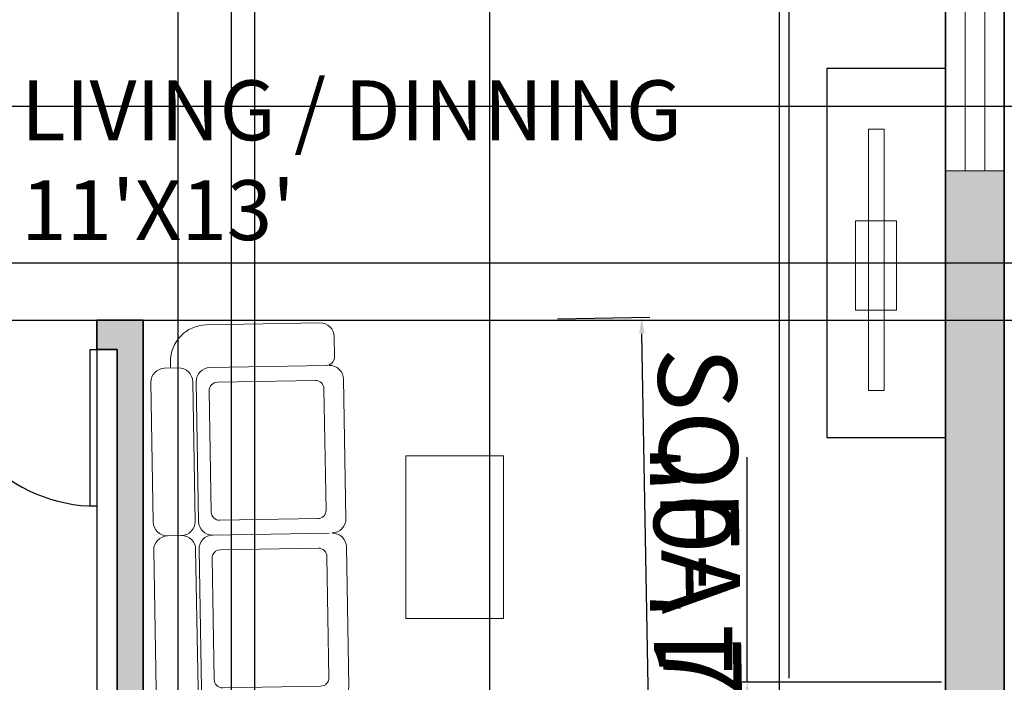
# Model space of a CAD drawing. Units: inches. Extents: x 1810 to 2254, y 313 to 1026.
# Tile 4 of 7: x 1988 to 2139, y 559 to 661. Entities that reach past the tile are written whole.
import ezdxf

# ---------------------------------------------------------------- set-up
doc = ezdxf.new("R2010")
doc.units = ezdxf.units.IN
for name, color, linetype, lineweight in [('A-ANNO-DIMS', 2, 'Continuous', 18), ('A-AREA-IDEN', 7, 'Continuous', 25), ('A-DOOR', 4, 'Continuous', 25), ('A-EQPM', 9, 'Continuous', 18), ('A-FLOR-CASE', 8, 'Continuous', 25), ('A-FURN', 8, 'Continuous', 18), ('A-GLAZ', 4, 'Continuous', 18), ('A-WALL', 7, 'Continuous', 35)]:
    doc.layers.add(name, color=color, linetype=linetype, lineweight=lineweight)
doc.layers.add('A-WALL-PATT', color=252, linetype='Continuous', lineweight=13, true_color=0x939598)
doc.styles.get("Standard").update_dxf_attribs({"font": 'arial.ttf'})
doc.dimstyles.new('ISO-25', dxfattribs={"dimtxt": 12, "dimasz": 2.5, "dimexe": 1.25, "dimexo": 0.625, "dimtad": 1, "dimdec": 1, "dimlunit": 4, "dimtxsty": 'Standard', "dimcen": 2.5, "dimadec": 0, "dimazin": 0, "dimtfac": 1, "dimtdec": 1, "dimtmove": 0, "dimatfit": 3, "dimfxl": 1, "dimarcsym": 0})

# ---------------------------------------------------------------- blocks, each defined once
blk = doc.blocks.new('A$C611E44E9')
for p, q in [((0.6611, 1.4447), (0.2101, 1.4447)), ((0.7111, 1.3223), (0.7111, 1.3947)), ((0.1084, 1.2927), (0.0584, 1.2927)), ((0.0584, 1.2924), (0.1084, 1.2924)), ((0.6811, 1.2924), (0.2205, 1.2924)), ((0.6811, 1.2924), (0.2205, 1.2924)), ((0.6811, 1.2922), (0.2205, 1.2922)), ((0.0084, 1.2424), (0.0084, 0.7424)), ((0.1584, 1.2424), (0.1584, 0.7424)), ((0.1705, 1.2422), (0.1705, 0.7424)), ((0.2465, 1.2392), (0.6374, 1.2392)), ((0.7418, 0.7424), (0.7418, 1.2422)), ((0.2165, 0.7749), (0.2165, 1.2092)), ((0.6674, 1.2092), (0.6674, 0.7749)), ((0.6374, 0.7449), (0.2465, 0.7449)), ((0.1224, 0.6827), (0.05, 0.6827)), ((0.1084, 0.6927), (0.0584, 0.6927)), ((0.0584, 0.6924), (0.1084, 0.6924)), ((0.2024, 0.6896), (0.7021, 0.6896)), ((0.6373, 0.6924), (0.2205, 0.6924)), ((0.6373, 0.6924), (0.2205, 0.6924)), ((0.8021, 0.6896), (1.3018, 0.6896)), ((1.4021, 0.6896), (1.9018, 0.6896)), ((0.1524, 0.6527), (0.1524, 0.2121)), ((1.982, 0.6589), (2.0543, 0.6589)), ((0, 0.6327), (0, 0.2017)), ((0.6691, 0.6192), (0.2348, 0.6192)), ((0.7521, 0.6289), (0.7521, 0.2121)), ((0.7521, 0.6289), (0.7521, 0.2121)), ((1.2688, 0.6192), (0.8345, 0.6192)), ((1.3521, 0.6289), (1.3521, 0.2121)), ((1.3521, 0.6289), (1.3521, 0.2121)), ((1.8688, 0.6192), (1.4345, 0.6192)), ((1.9518, 0.6289), (1.9518, 0.2121)), ((1.952, 0.6289), (1.952, 0.2121)), ((2.1043, 0.6089), (2.1043, 0.2017)), ((0.2048, 0.5892), (0.2048, 0.2381)), ((0.6991, 0.2381), (0.6991, 0.5892)), ((0.8045, 0.5892), (0.8045, 0.2381)), ((1.2988, 0.2381), (1.2988, 0.5892)), ((1.4045, 0.5892), (1.4045, 0.2381)), ((1.8988, 0.2381), (1.8988, 0.5892)), ((0.2348, 0.2081), (0.6691, 0.2081)), ((0.8345, 0.2081), (1.2688, 0.2081)), ((1.4345, 0.2081), (1.8688, 0.2081)), ((0.7021, 0.1621), (0.2024, 0.1621)), ((0.7024, 0.15), (0.2024, 0.15)), ((1.3018, 0.1621), (0.8021, 0.1621)), ((1.3021, 0.15), (0.8021, 0.15)), ((1.9018, 0.1621), (1.4021, 0.1621)), ((1.9021, 0.15), (1.4021, 0.15)), ((0.13, 0.0717), (0.15, 0.0717)), ((0.1524, 0.05), (0.1524, 0.1)), ((0.7521, 0.05), (0.7521, 0.1)), ((0.7524, 0.1), (0.7524, 0.05)), ((1.3521, 0.05), (1.3521, 0.1)), ((1.3524, 0.1), (1.3524, 0.05)), ((1.952, 0.05), (1.952, 0.1)), ((1.9521, 0.1), (1.9521, 0.05)), ((1.9743, 0.0717), (1.9543, 0.0717)), ((0.7024, 0), (0.2024, 0)), ((1.3021, 0), (0.8021, 0)), ((1.9021, 0), (1.4021, 0))]:
    blk.add_line(p, q)
for centre, radius, start, end in [((0.2101, 1.3147), 0.13, 90, 189.8614), ((0.6611, 1.3947), 0.05, 0, 90), ((0.6811, 1.3223), 0.03, 270, 0), ((0.0584, 1.2424), 0.05, 90, 180), ((0.1084, 1.2424), 0.05, 0, 90), ((0.2205, 1.2422), 0.05, 90, 180), ((0.6918, 1.2422), 0.05, 0, 90), ((0.2465, 1.2092), 0.03, 90, 180), ((0.6374, 1.2092), 0.03, 0, 90), ((0.0584, 0.7424), 0.05, 180, 270), ((0.1084, 0.7424), 0.05, 270, 0), ((0.2205, 0.7424), 0.05, 180, 270), ((0.2465, 0.7749), 0.03, 180, 270), ((0.6374, 0.7749), 0.03, 270, 0), ((0.653, 0.796), 0.1037, 267.2489, 328.8794), ((0.05, 0.6327), 0.05, 90, 180), ((0.1224, 0.6527), 0.03, 0, 90), ((0.1981, 0.6441), 0.0458, 84.6649, 178.9903), ((0.7021, 0.6396), 0.05, 0, 90), ((0.8021, 0.6396), 0.05, 90, 180), ((1.3018, 0.6396), 0.05, 0, 90), ((1.4021, 0.6396), 0.05, 90, 180), ((1.9018, 0.6396), 0.05, 0, 90), ((1.982, 0.6289), 0.03, 90, 180), ((2.0543, 0.6089), 0.05, 0, 90), ((0.2348, 0.5892), 0.03, 90, 180), ((0.6691, 0.5892), 0.03, 0, 90), ((0.8345, 0.5892), 0.03, 90, 180), ((1.2688, 0.5892), 0.03, 0, 90), ((1.4345, 0.5892), 0.03, 90, 180), ((1.8688, 0.5892), 0.03, 0, 90), ((0.2024, 0.2121), 0.05, 180, 270), ((0.2348, 0.2381), 0.03, 180, 270), ((0.6691, 0.2381), 0.03, 270, 0), ((0.7021, 0.2121), 0.05, 270, 0), ((0.8021, 0.2121), 0.05, 180, 270), ((0.8345, 0.2381), 0.03, 180, 270), ((1.2688, 0.2381), 0.03, 270, 0), ((1.3018, 0.2121), 0.05, 270, 0), ((1.4021, 0.2121), 0.05, 180, 270), ((1.4345, 0.2381), 0.03, 180, 270), ((1.8688, 0.2381), 0.03, 270, 0), ((1.9018, 0.2121), 0.05, 270, 0), ((0.13, 0.2017), 0.13, 180, 270), ((1.9743, 0.2017), 0.13, 270, 0), ((0.2024, 0.1), 0.05, 90, 180), ((0.7024, 0.1), 0.05, 0, 90), ((0.8021, 0.1), 0.05, 90, 180), ((1.3021, 0.1), 0.05, 0, 90), ((1.4021, 0.1), 0.05, 90, 180), ((1.9021, 0.1), 0.05, 0, 90), ((0.2024, 0.05), 0.05, 180, 270), ((0.7024, 0.05), 0.05, 270, 0), ((0.8021, 0.05), 0.05, 180, 270), ((1.3021, 0.05), 0.05, 270, 0), ((1.4021, 0.05), 0.05, 180, 270), ((1.9021, 0.05), 0.05, 270, 0)]:
    blk.add_arc(centre, radius, start, end)
blk = doc.blocks.new('*U16')
for p, q in [((0, 0), (0, -6)), ((40, 0), (40, -6))]:
    blk.add_line(p, q)
blk.add_lwpolyline([(0, 0), (0, 40), (1.75, 40), (1.75, 0)], close=True)
blk.add_arc((0, 0), 40, 0, 90)
blk = doc.blocks.new('*D23')
at = {"layer": 'A-ANNO-DIMS', "color": 0, "lineweight": -2, "transparency": 16777216}
for p, q in [((2130.99, 851.61), (2253.63, 851.61)), ((2252.38, 849.11), (2252.38, 437.11)), ((2130.99, 434.61), (2253.63, 434.61))]:
    blk.add_line(p, q, dxfattribs=at)
at = {"layer": 'A-ANNO-DIMS', "color": 0, "transparency": 16777216}
for points in [[(2251.96, 849.11), (2252.8, 849.11), (2252.38, 851.61)], [(2251.96, 437.11), (2252.8, 437.11), (2252.38, 434.61)]]:
    blk.add_solid(points, dxfattribs=at)
at = {"layer": 'Defpoints', "color": 0, "transparency": 16777216}
for p in [(2130.36, 851.61), (2130.36, 434.61), (2252.38, 434.61)]:
    blk.add_point(p, dxfattribs=at)
at = {"layer": 'A-ANNO-DIMS', "color": 0, "transparency": 16777216, "insert": (2245.62, 643.11), "char_height": 12, "attachment_point": 5, "rotation": 90}
blk.add_mtext('34\'-9"', dxfattribs=at)
blk = doc.blocks.new('WIN-36IN-WALL9')
for p, q in [((0, 9), (0, 0)), ((36, 9), (36, 0)), ((0, 6), (36, 6)), ((0, 3), (36, 3))]:
    blk.add_line(p, q)
blk = doc.blocks.new('*D44')
at = {"layer": 'A-ANNO-DIMS', "color": 0, "lineweight": -2, "transparency": 16777216}
for p, q in [((2070.88, 614.82), (2085.02, 615.06)), ((2085.29, 527.43), (2083.81, 612.54)), ((2072.44, 524.71), (2086.58, 524.96))]:
    blk.add_line(p, q, dxfattribs=at)
at = {"layer": 'A-ANNO-DIMS', "color": 0, "transparency": 16777216}
for points in [[(2084.23, 612.55), (2083.4, 612.54), (2083.77, 615.04)], [(2085.7, 527.44), (2084.87, 527.43), (2085.33, 524.93)]]:
    blk.add_solid(points, dxfattribs=at)
at = {"layer": 'Defpoints', "color": 0, "transparency": 16777216}
for p in [(2070.25, 614.81), (2083.77, 615.04), (2071.81, 524.7)]:
    blk.add_point(p, dxfattribs=at)
at = {"layer": 'A-ANNO-DIMS', "color": 0, "transparency": 16777216, "insert": (2091.38, 570.11), "char_height": 12, "attachment_point": 5, "rotation": 270.9916}
blk.add_mtext('SOFA 7\'-6"', dxfattribs=at)
blk = doc.blocks.new('*D54')
at = {"layer": 'A-ANNO-DIMS', "color": 0, "lineweight": -2, "transparency": 16777216}
for p, q in [((2130.99, 715.11), (2162.01, 715.11)), ((2160.76, 712.61), (2160.76, 676.02)), ((2130.99, 673.52), (2162.01, 673.52)), ((2160.76, 673.52), (2160.76, 609.92))]:
    blk.add_line(p, q, dxfattribs=at)
at = {"layer": 'A-ANNO-DIMS', "color": 0, "transparency": 16777216}
for points in [[(2160.35, 712.61), (2161.18, 712.61), (2160.76, 715.11)], [(2160.35, 676.02), (2161.18, 676.02), (2160.76, 673.52)]]:
    blk.add_solid(points, dxfattribs=at)
at = {"layer": 'Defpoints', "color": 0, "transparency": 16777216}
for p in [(2130.36, 715.11), (2130.36, 673.52), (2160.76, 673.52)]:
    blk.add_point(p, dxfattribs=at)
at = {"layer": 'A-ANNO-DIMS', "color": 0, "transparency": 16777216, "insert": (2153.93, 640.47), "char_height": 12, "attachment_point": 5, "rotation": 90}
blk.add_mtext('3\'-5 1/2"', dxfattribs=at)
blk = doc.blocks.new('*D57')
at = {"layer": 'A-ANNO-DIMS', "color": 0, "lineweight": -2, "transparency": 16777216}
for p, q in [((2104.86, 718.99), (2104.86, 323.71)), ((2130.36, 718.99), (2130.36, 323.71)), ((2107.36, 324.96), (2127.86, 324.96)), ((2130.36, 324.96), (2194.18, 324.96))]:
    blk.add_line(p, q, dxfattribs=at)
at = {"layer": 'A-ANNO-DIMS', "color": 0, "transparency": 16777216}
for points in [[(2107.36, 325.38), (2107.36, 324.55), (2104.86, 324.96)], [(2127.86, 325.38), (2127.86, 324.55), (2130.36, 324.96)]]:
    blk.add_solid(points, dxfattribs=at)
at = {"layer": 'Defpoints', "color": 0, "transparency": 16777216}
for p in [(2104.86, 719.61), (2130.36, 719.61), (2130.36, 324.96)]:
    blk.add_point(p, dxfattribs=at)
at = {"layer": 'A-ANNO-DIMS', "color": 0, "transparency": 16777216, "insert": (2163.52, 331.79), "char_height": 12, "attachment_point": 5}
blk.add_mtext('2\'-1 1/2"', dxfattribs=at)
blk = doc.blocks.new('*D59')
at = {"layer": 'A-ANNO-DIMS', "color": 0, "lineweight": -2, "transparency": 16777216}
for p, q in [((2024.44, 714.49), (2024.44, 323.71)), ((2060.44, 714.49), (2060.44, 323.71)), ((2026.94, 324.96), (2057.94, 324.96))]:
    blk.add_line(p, q, dxfattribs=at)
at = {"layer": 'A-ANNO-DIMS', "color": 0, "transparency": 16777216}
for points in [[(2026.94, 325.38), (2026.94, 324.55), (2024.44, 324.96)], [(2057.94, 325.38), (2057.94, 324.55), (2060.44, 324.96)]]:
    blk.add_solid(points, dxfattribs=at)
at = {"layer": 'Defpoints', "color": 0, "transparency": 16777216}
for p in [(2024.44, 715.11), (2060.44, 715.11), (2060.44, 324.96)]:
    blk.add_point(p, dxfattribs=at)
at = {"layer": 'A-ANNO-DIMS', "color": 0, "transparency": 16777216, "insert": (2042.44, 331.72), "char_height": 12, "attachment_point": 5}
blk.add_mtext('3\'-0"', dxfattribs=at)
blk = doc.blocks.new('*D61')
at = {"layer": 'A-ANNO-DIMS', "color": 0, "lineweight": -2, "transparency": 16777216}
for p, q in [((2106.36, 559.74), (2106.36, 892.26)), ((2130.36, 559.74), (2130.36, 892.26)), ((2108.86, 891.01), (2127.86, 891.01)), ((2130.36, 891.01), (2166.22, 891.01))]:
    blk.add_line(p, q, dxfattribs=at)
at = {"layer": 'A-ANNO-DIMS', "color": 0, "transparency": 16777216}
for points in [[(2108.86, 891.43), (2108.86, 890.6), (2106.36, 891.01)], [(2127.86, 891.43), (2127.86, 890.6), (2130.36, 891.01)]]:
    blk.add_solid(points, dxfattribs=at)
at = {"layer": 'Defpoints', "color": 0, "transparency": 16777216}
for p in [(2130.36, 891.01), (2106.36, 559.11), (2130.36, 559.11)]:
    blk.add_point(p, dxfattribs=at)
at = {"layer": 'A-ANNO-DIMS', "color": 0, "transparency": 16777216, "insert": (2149.54, 897.76), "char_height": 12, "attachment_point": 5}
blk.add_mtext('2\'-0"', dxfattribs=at)
blk = doc.blocks.new('*D63')
at = {"layer": 'A-ANNO-DIMS', "color": 0, "lineweight": -2, "transparency": 16777216}
for p, q in [((2169.76, 679.36), (2169.76, 715.21)), ((1973.49, 679.36), (2171.01, 679.36)), ((2169.76, 649.92), (2169.76, 676.86)), ((1973.49, 647.42), (2171.01, 647.42))]:
    blk.add_line(p, q, dxfattribs=at)
at = {"layer": 'A-ANNO-DIMS', "color": 0, "transparency": 16777216}
for points in [[(2169.35, 676.86), (2170.18, 676.86), (2169.76, 679.36)], [(2169.35, 649.92), (2170.18, 649.92), (2169.76, 647.42)]]:
    blk.add_solid(points, dxfattribs=at)
at = {"layer": 'Defpoints', "color": 0, "transparency": 16777216}
for p in [(1972.86, 679.36), (2169.76, 679.36), (1972.86, 647.42)]:
    blk.add_point(p, dxfattribs=at)
at = {"layer": 'A-ANNO-DIMS', "color": 0, "transparency": 16777216, "insert": (2163.01, 698.54), "char_height": 12, "attachment_point": 5, "rotation": 90}
blk.add_mtext('2\'-8"', dxfattribs=at)
blk = doc.blocks.new('*D64')
at = {"layer": 'A-ANNO-DIMS', "color": 0, "lineweight": -2, "transparency": 16777216}
for p, q in [((2169.76, 623.42), (2169.76, 659.07)), ((1973.49, 623.42), (2171.01, 623.42)), ((2169.76, 617.11), (2169.76, 620.92)), ((1973.49, 614.61), (2171.01, 614.61))]:
    blk.add_line(p, q, dxfattribs=at)
at = {"layer": 'A-ANNO-DIMS', "color": 0, "transparency": 16777216}
for points in [[(2169.35, 620.92), (2170.18, 620.92), (2169.76, 623.42)], [(2169.35, 617.11), (2170.18, 617.11), (2169.76, 614.61)]]:
    blk.add_solid(points, dxfattribs=at)
at = {"layer": 'Defpoints', "color": 0, "transparency": 16777216}
for p in [(1972.86, 623.42), (2169.76, 623.42), (1972.86, 614.61)]:
    blk.add_point(p, dxfattribs=at)
at = {"layer": 'A-ANNO-DIMS', "color": 0, "transparency": 16777216, "insert": (2163.01, 642.49), "char_height": 12, "attachment_point": 5, "rotation": 90}
blk.add_mtext('0\'-9"', dxfattribs=at)
blk = doc.blocks.new('*D66')
at = {"layer": 'A-ANNO-DIMS', "color": 0, "lineweight": -2, "transparency": 16777216}
for p, q in [((1976.27, 609.49), (1976.27, 323.71)), ((2000.27, 609.49), (2000.27, 323.71)), ((1978.77, 324.96), (1997.77, 324.96)), ((2000.27, 324.96), (2036.12, 324.96))]:
    blk.add_line(p, q, dxfattribs=at)
at = {"layer": 'A-ANNO-DIMS', "color": 0, "transparency": 16777216}
for points in [[(1978.77, 325.38), (1978.77, 324.55), (1976.27, 324.96)], [(1997.77, 325.38), (1997.77, 324.55), (2000.27, 324.96)]]:
    blk.add_solid(points, dxfattribs=at)
at = {"layer": 'Defpoints', "color": 0, "transparency": 16777216}
for p in [(1976.27, 610.11), (2000.27, 610.11), (2000.27, 324.96)]:
    blk.add_point(p, dxfattribs=at)
at = {"layer": 'A-ANNO-DIMS', "color": 0, "transparency": 16777216, "insert": (2019.45, 331.72), "char_height": 12, "attachment_point": 5}
blk.add_mtext('2\'-0"', dxfattribs=at)
blk = doc.blocks.new('*D67')
at = {"layer": 'A-ANNO-DIMS', "color": 0, "lineweight": -2, "transparency": 16777216}
for p, q in [((1976.68, 714.49), (1976.68, 323.71)), ((2012.68, 714.49), (2012.68, 323.71)), ((1979.18, 324.96), (2010.18, 324.96))]:
    blk.add_line(p, q, dxfattribs=at)
at = {"layer": 'A-ANNO-DIMS', "color": 0, "transparency": 16777216}
for points in [[(1979.18, 325.38), (1979.18, 324.55), (1976.68, 324.96)], [(2010.18, 325.38), (2010.18, 324.55), (2012.68, 324.96)]]:
    blk.add_solid(points, dxfattribs=at)
at = {"layer": 'Defpoints', "color": 0, "transparency": 16777216}
for p in [(1976.68, 715.11), (2012.68, 715.11), (2012.68, 324.96)]:
    blk.add_point(p, dxfattribs=at)
at = {"layer": 'A-ANNO-DIMS', "color": 0, "transparency": 16777216, "insert": (1994.68, 331.72), "char_height": 12, "attachment_point": 5}
blk.add_mtext('3\'-0"', dxfattribs=at)
blk = doc.blocks.new('*D68')
at = {"layer": 'A-ANNO-DIMS', "color": 0, "lineweight": -2, "transparency": 16777216}
for p, q in [((2020.86, 826.99), (2020.86, 323.71)), ((2104.86, 826.99), (2104.86, 323.71)), ((2023.36, 324.96), (2102.36, 324.96))]:
    blk.add_line(p, q, dxfattribs=at)
at = {"layer": 'A-ANNO-DIMS', "color": 0, "transparency": 16777216}
for points in [[(2023.36, 325.38), (2023.36, 324.55), (2020.86, 324.96)], [(2102.36, 325.38), (2102.36, 324.55), (2104.86, 324.96)]]:
    blk.add_solid(points, dxfattribs=at)
at = {"layer": 'Defpoints', "color": 0, "transparency": 16777216}
for p in [(2020.86, 827.61), (2104.86, 827.61), (2104.86, 324.96)]:
    blk.add_point(p, dxfattribs=at)
at = {"layer": 'A-ANNO-DIMS', "color": 0, "transparency": 16777216, "insert": (2062.86, 331.72), "char_height": 12, "attachment_point": 5}
blk.add_mtext('7\'-0"', dxfattribs=at)
blk = doc.blocks.new('*D75')
at = {"layer": 'A-ANNO-DIMS', "color": 0, "lineweight": -2, "transparency": 16777216}
for p, q in [((2099.96, 559.11), (2099.96, 593.63)), ((2129.74, 559.11), (2098.71, 559.11)), ((2099.96, 549.61), (2099.96, 556.61)), ((2129.74, 547.11), (2098.71, 547.11))]:
    blk.add_line(p, q, dxfattribs=at)
at = {"layer": 'A-ANNO-DIMS', "color": 0, "transparency": 16777216}
for points in [[(2099.55, 556.61), (2100.38, 556.61), (2099.96, 559.11)], [(2099.55, 549.61), (2100.38, 549.61), (2099.96, 547.11)]]:
    blk.add_solid(points, dxfattribs=at)
at = {"layer": 'Defpoints', "color": 0, "transparency": 16777216}
for p in [(2099.96, 559.11), (2130.36, 559.11), (2130.36, 547.11)]:
    blk.add_point(p, dxfattribs=at)
at = {"layer": 'A-ANNO-DIMS', "color": 0, "transparency": 16777216, "insert": (2093.21, 577.62), "char_height": 12, "attachment_point": 5, "rotation": 90}
blk.add_mtext('1\'-0"', dxfattribs=at)

msp = doc.modelspace()

# ---------------------------------------------------------------- hatches: boundary and pattern name
at = {"layer": 'A-WALL-PATT'}
h = msp.add_hatch(color=256, dxfattribs=at)
h.dxf.hatch_style = 1
h.paths.add_polyline_path([(1943.78, 860.61), (1875.36, 860.61), (1875.36, 706.11), (1884.36, 706.11), (1884.36, 715.11), (1968.36, 715.11), (1968.36, 703.36), (1971.96, 703.36), (1972.86, 703.36), (1972.86, 715.11), (1976.68, 715.11), (1976.68, 719.61), (1884.36, 719.61), (1884.36, 851.61), (1943.73, 851.61)])
h.paths.add_polyline_path([(2048.15, 860.61), (1979.78, 860.61), (1979.73, 851.61), (2016.36, 851.61), (2016.36, 719.61), (2012.68, 719.61), (2012.68, 716.01), (2012.68, 715.11), (2024.44, 715.11), (2024.44, 719.61), (2020.86, 719.61), (2020.86, 851.61), (2048.15, 851.61)])
h.paths.add_polyline_path([(2139.36, 860.61), (2084.15, 860.61), (2084.15, 851.61), (2130.36, 851.61), (2130.36, 719.61), (2060.44, 719.61), (2060.44, 716.01), (2060.44, 715.11), (2130.36, 715.11), (2130.36, 673.52), (2139.36, 673.52)])
h.paths.add_polyline_path([(1884.36, 682.11), (1875.36, 682.11), (1875.36, 654.79), (1884.36, 654.79), (1884.36, 662.61), (1968.36, 662.61), (1968.36, 647.42), (1971.96, 647.42), (1972.86, 647.42), (1972.86, 679.36), (1968.36, 679.36), (1968.36, 667.11), (1884.36, 667.11)])
h.paths.add_polyline_path([(1884.36, 610.11), (1972.86, 610.11), (1976.27, 610.11), (1976.27, 614.61), (1972.86, 614.61), (1972.86, 623.42), (1968.36, 623.42), (1968.36, 614.61), (1884.36, 614.61), (1884.36, 630.79), (1875.36, 630.79), (1875.36, 481.11), (1939.68, 481.11), (1939.68, 490.11), (1884.36, 490.11)])
h.paths.add_polyline_path([(2007.36, 518.61), (2038.86, 518.61), (2038.86, 494.59), (2043.36, 494.59), (2043.36, 518.61), (2070.36, 518.61), (2070.36, 523.11), (2007.36, 523.11), (2007.36, 614.61), (2000.27, 614.61), (2000.27, 610.11), (2003.36, 610.11), (2003.36, 490.11), (1975.68, 490.11), (1975.68, 481.11), (2007.36, 481.11)])
h.paths.add_polyline_path([(2139.36, 637.52), (2130.36, 637.52), (2130.36, 434.61), (2043.36, 434.61), (2043.36, 458.59), (2038.86, 458.59), (2038.86, 434.61), (2035.41, 434.61), (2035.41, 431.01), (2035.41, 425.61), (2139.36, 425.61)])

# ---------------------------------------------------------------- linework, layer by layer
at = {"layer": 'A-EQPM'}
for points in [[(2118.55, 643.88), (2120.94, 643.88), (2120.94, 603.82), (2118.55, 603.82)], [(2116.54, 629.82), (2122.82, 629.82), (2122.82, 616.13), (2116.54, 616.13)]]:
    msp.add_lwpolyline(points, close=True, dxfattribs=at)
at = {"layer": 'A-FLOR-CASE'}
for p, q in [((2130.36, 653.18), (2112.14, 653.18)), ((2112.14, 653.18), (2112.14, 596.66)), ((2112.14, 596.66), (2130.36, 596.66))]:
    msp.add_line(p, q, dxfattribs=at)
at = {"layer": 'A-FURN'}
for p, q in [((2047.65, 593.8), (2047.65, 568.9)), ((2062.61, 593.8), (2047.65, 593.8)), ((2062.61, 568.9), (2062.61, 593.8)), ((2047.65, 568.9), (2062.61, 568.9))]:
    msp.add_line(p, q, dxfattribs=at)
at = {"layer": 'A-WALL'}
for p, q in [((2139.36, 860.61), (2139.36, 425.61)), ((2130.36, 715.11), (2130.36, 434.61)), ((2000.27, 614.61), (2007.36, 614.61)), ((2000.27, 614.61), (2000.27, 610.11)), ((2007.36, 614.61), (2007.36, 523.11)), ((2000.27, 610.11), (2003.36, 610.11)), ((2003.36, 610.11), (2003.36, 490.11))]:
    msp.add_line(p, q, dxfattribs=at)

# ---------------------------------------------------------------- block references
at = {"layer": 'A-DOOR', "xscale": 0.6, "yscale": 0.6, "zscale": 0.6, "rotation": 180}
msp.add_blockref('*U16', (2000.27, 610.11), dxfattribs=at)
at = {"layer": 'A-FURN', "xscale": -42.82681931732404, "yscale": 42.82681931732404, "zscale": 42.82681931732404, "rotation": 270.9915511878509}
msp.add_blockref('A$C611E44E9', (2009.95, 523.63), dxfattribs=at)
at = {"layer": 'A-GLAZ', "rotation": 89.99999999999984}
msp.add_blockref('WIN-36IN-WALL9', (2139.36, 637.52), dxfattribs=at)

# ---------------------------------------------------------------- texts
at = {"layer": 'A-AREA-IDEN', "insert": (1988.67, 651.38), "char_height": 9.1812, "attachment_point": 1}
msp.add_mtext_dynamic_manual_height_columns("LIVING / DINNING\\P11'X13'", width=133.5247, gutter_width=45.91, heights=[0], dxfattribs=at)

# ---------------------------------------------------------------- dimensions: what is measured, and where the dimension line sits
at = {"layer": 'A-ANNO-DIMS'}
for base, p1, p2, picture, middle in [((2130.36, 891.01), (2106.36, 559.11), (2130.36, 559.11), '*D61', (2149.54, 897.76)), ((2104.86, 324.96), (2020.86, 827.61), (2104.86, 827.61), '*D68', (2062.86, 331.72)), ((2130.36, 324.96), (2104.86, 719.61), (2130.36, 719.61), '*D57', (2163.52, 331.79)), ((2012.68, 324.96), (1976.68, 715.11), (2012.68, 715.11), '*D67', (1994.68, 331.72)), ((2060.44, 324.96), (2024.44, 715.11), (2060.44, 715.11), '*D59', (2042.44, 331.72)), ((2000.27, 324.96), (1976.27, 610.11), (2000.27, 610.11), '*D66', (2019.45, 331.72))]:
    dim = msp.add_linear_dim(base=base, p1=p1, p2=p2, dimstyle='ISO-25', override={"dimdec": 1, "dimlfac": 1, "dimrnd": 0, "dimzin": 1, "dimdsep": 46, "dimlunit": 4, "dimfrac": 2}, dxfattribs=at)
    dim.commit()
    dim.dimension.update_dxf_attribs({"geometry": picture, "text_midpoint": middle})
for base, p1, p2, angle, override, picture, middle in [((2252.38, 434.61), (2130.36, 851.61), (2130.36, 434.61), 90, {"dimclrd": 0, "dimclre": 0, "dimclrt": 0}, '*D23', (2245.62, 643.11)), ((2169.76, 679.36), (1972.86, 647.42), (1972.86, 679.36), 90, {"dimdec": 1, "dimlfac": 1, "dimrnd": 0, "dimzin": 1, "dimdsep": 46, "dimlunit": 4, "dimfrac": 2}, '*D63', (2163.01, 698.54)), ((2160.76, 673.52), (2130.36, 715.11), (2130.36, 673.52), 270, {"dimdec": 1, "dimlfac": 1, "dimrnd": 0, "dimzin": 1, "dimdsep": 46, "dimlunit": 4, "dimfrac": 2}, '*D54', (2153.93, 640.47)), ((2169.76, 623.42), (1972.86, 614.61), (1972.86, 623.42), 90, {"dimdec": 1, "dimlfac": 1, "dimrnd": 0, "dimzin": 1, "dimdsep": 46, "dimlunit": 4, "dimfrac": 2}, '*D64', (2163.01, 642.49)), ((2099.96, 559.11), (2130.36, 547.11), (2130.36, 559.11), 90, {"dimdec": 1, "dimlfac": 1, "dimrnd": 0, "dimzin": 1, "dimdsep": 46, "dimlunit": 4, "dimfrac": 2}, '*D75', (2093.21, 577.62))]:
    dim = msp.add_linear_dim(base=base, p1=p1, p2=p2, angle=angle, dimstyle='ISO-25', override=override, dxfattribs=at)
    dim.commit()
    dim.dimension.update_dxf_attribs({"geometry": picture, "text_midpoint": middle})
dim = msp.add_linear_dim(base=(2083.77, 615.04), p1=(2071.81, 524.7), p2=(2070.25, 614.81), angle=90.9916, text='SOFA <>', dimstyle='ISO-25', override={"dimdec": 1, "dimlfac": 1, "dimrnd": 0, "dimzin": 1, "dimdsep": 46, "dimlunit": 4, "dimfrac": 2}, dxfattribs=at)
dim.commit()
dim.dimension.update_dxf_attribs({"geometry": '*D44', "text_midpoint": (2091.38, 570.11)})

doc.saveas('drawing.dxf')
